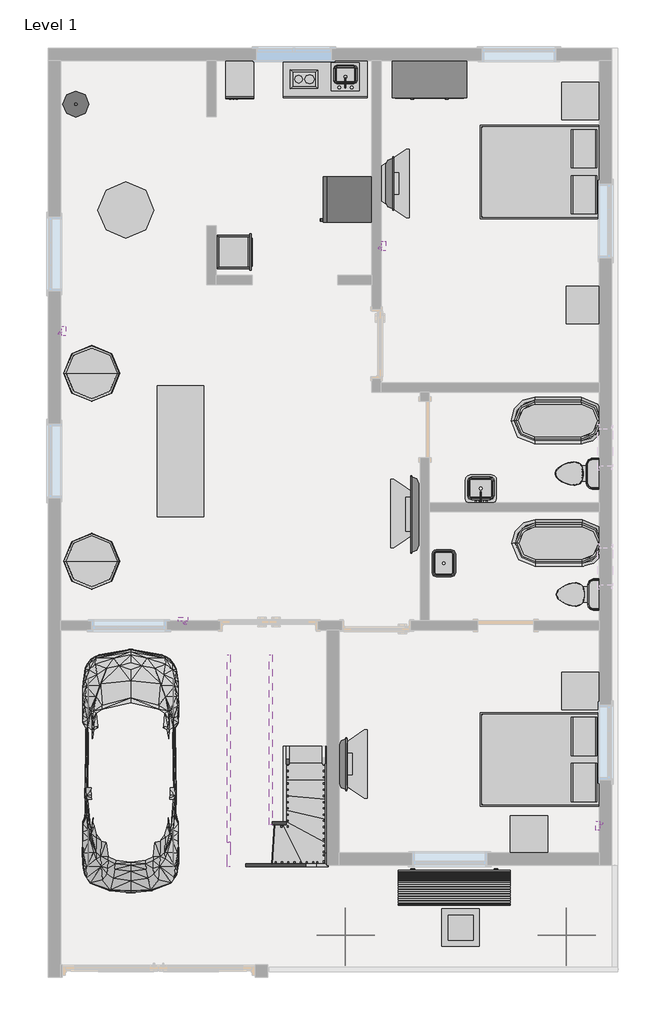
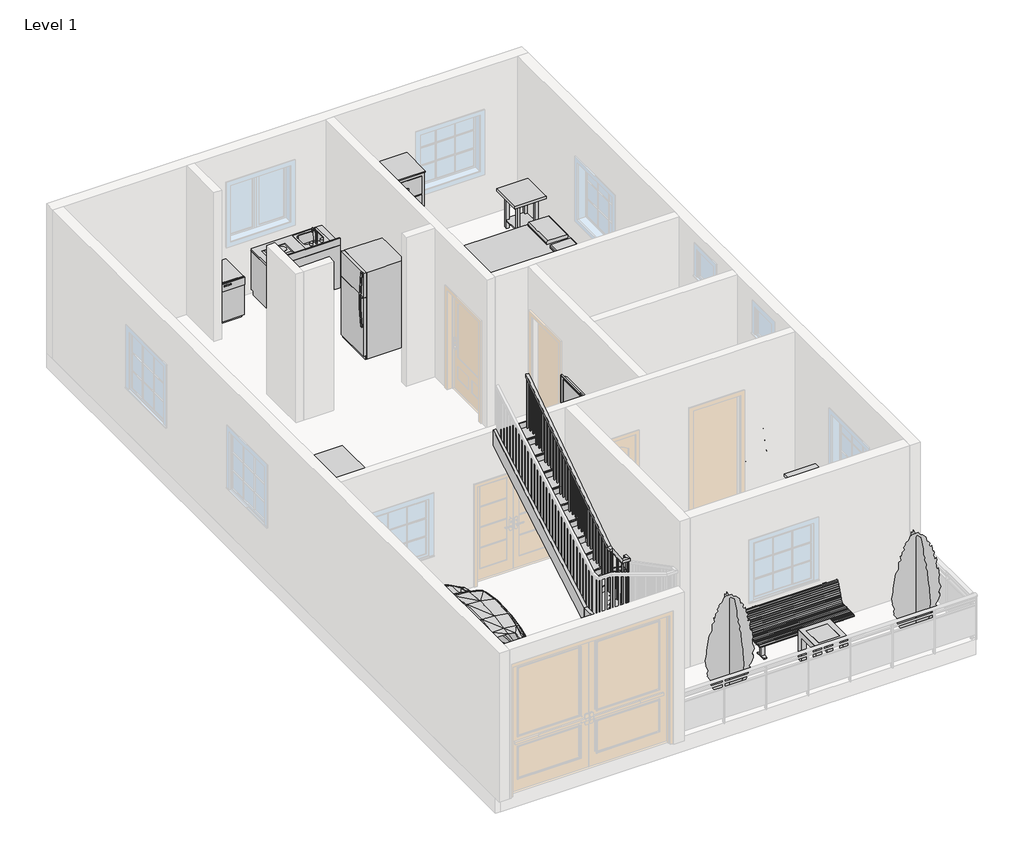
# One storey, part 3 of 3: 19 furniture elements, 10 proxies, 9 members, 8 flow terminals, 3 geographic elements, 1 railing, 1 stair flight.
"""IFC4 building model written with IfcOpenShell, lengths in millimetres."""

from ifc_helpers import new_model, si_unit, frame, origin, place, context, project, spatial, polyline, outline, extrude, faceted_brep, transform, mapped, element, save
from components import proxy_7e1014cc, proxy_fe84b772, proxy_844211aa, proxy_8b8c2dc4, rpc_beetle_rpc_beetle_3ce7ba48, rpc_picture_frame_rpc_picture_frame_c25e3fe9, proxy_a13a33b2, flow_terminal_871c2e40, flow_terminal_d49f872f, flow_terminal_62a433f7, toilet_domestic_3d_toilet_domestic_3d_f7549cf7, toilet_domestic_3d_toilet_domestic_3d_183bbd19, flow_terminal_b374fae2, furniture_1d2926bd, furniture_95afb093, furniture_9fa109b2, furniture_56245f3a, furniture_fdf74506, tv_stand_tv_stand_6ce107e5, furniture_b5c51a22, furniture_92191dda, furniture_905aceb5, furniture_5bc9ed15, furniture_c80d6d9c, geographic_element_235d1464, rpc_tree_conifer_chinese_juniper_7_1b9786cd, stair_flight_e7e63c14

model = new_model("IFC4")

# Units and contexts
model_context = context("Model", 3, world=origin())
ifc_project = project(units=[si_unit("LENGTHUNIT", "METRE", prefix="MILLI")], contexts=[model_context])

# Site, building, storey
site = spatial("IfcSite", under=ifc_project)
building = spatial("IfcBuilding", under=site)
storey = spatial("IfcBuildingStorey", under=building, Name="Level 1", Elevation=0.0)

# Proxies
placement = place(None, origin())
proxy_shape = proxy_7e1014cc(model_context)
element("IfcBuildingElementProxy", 1, Name="18\" x 24\" x 34 1/2\"", ObjectType="18\" x 24\" x 34 1/2\"", at=placement, inside=storey, context=model_context, shape_type="MappedRepresentation", body=[
    mapped(proxy_shape, transform((-12711.8273955, 12635.8692234, 0.0), x_axis=(1.0, 0.0, 0.0), y_axis=(0.0, 1.0, 0.0), z_axis=(0.0, 0.0, 1.0))),
])
proxy_2_shape = proxy_fe84b772(model_context)
element("IfcBuildingElementProxy", 2, Name="Cook Top-2 Unit : 12\" x 18\"", ObjectType="Cook Top-2 Unit : 12\" x 18\"", at=placement, inside=storey, context=model_context, shape_type="MappedRepresentation", body=[
    mapped(proxy_2_shape, transform((-11381.8347226, 12978.5187882, 0.0), x_axis=(0.0, -1.0000000000000002, 0.0), y_axis=(1.0000000000000002, 0.0, 0.0), z_axis=(0.0, 0.0, 1.0))),
])
proxy_3_shape = proxy_844211aa(model_context)
element("IfcBuildingElementProxy", 3, Name="Kitchenette - Small : 54\"", ObjectType="Kitchenette - Small : 54\"", at=placement, inside=storey, context=model_context, shape_type="MappedRepresentation", body=[
    mapped(proxy_3_shape, transform((-10989.9722221, 12597.5187882, 0.0), x_axis=(-1.0000000000000002, 0.0, 0.0), y_axis=(0.0, -1.0000000000000002, 0.0), z_axis=(0.0, 0.0, 1.0))),
])
proxy_4_shape = proxy_8b8c2dc4(model_context)
element("IfcBuildingElementProxy", 4, Name="Oven Double-Built-in : 21 1/2\" x 39 1/4\" x 21\"", ObjectType="Oven Double-Built-in : 21 1/2\" x 39 1/4\" x 21\"", at=placement, inside=storey, context=model_context, shape_type="MappedRepresentation", body=[
    mapped(proxy_4_shape, transform((-12366.2440681, 10118.0937155, 0.0), x_axis=(0.0, 1.0000000000000009, 0.0), y_axis=(-1.0000000000000009, 0.0, 0.0), z_axis=(0.0, 0.0, 1.0))),
])
rpc_beetle_rpc_beetle_shape = rpc_beetle_rpc_beetle_3ce7ba48(model_context)
element("IfcBuildingElementProxy", 5, Name="RPC Beetle : RPC Beetle", ObjectType="RPC Beetle : RPC Beetle", at=placement, inside=storey, context=model_context, shape_type="MappedRepresentation", body=[
    mapped(rpc_beetle_rpc_beetle_shape, transform((-14183.709927, 380.1187882, 0.0), x_axis=(1.0, 0.0, 0.0), y_axis=(0.0, 1.0, 0.0), z_axis=(0.0, 0.0, 1.0))),
])
rpc_picture_frame_rpc_picture_frame_shape = rpc_picture_frame_rpc_picture_frame_c25e3fe9(model_context)
element("IfcBuildingElementProxy", 6, Name="RPC Picture Frame : RPC Picture Frame", ObjectType="RPC Picture Frame : RPC Picture Frame", at=placement, inside=storey, context=model_context, shape_type="MappedRepresentation", body=[
    mapped(rpc_picture_frame_rpc_picture_frame_shape, transform((-10081.609927, 10181.9106753, 1828.8), x_axis=(0.0, 1.0000000000000002, 0.0), y_axis=(-1.0000000000000002, 0.0, 0.0), z_axis=(0.0, 0.0, 1.0))),
])
element("IfcBuildingElementProxy", 7, Name="RPC Picture Frame : RPC Picture Frame", ObjectType="RPC Picture Frame : RPC Picture Frame", at=placement, inside=storey, context=model_context, shape_type="MappedRepresentation", body=[
    mapped(rpc_picture_frame_rpc_picture_frame_shape, transform((-13328.659788, 4063.1187882, 1828.8), x_axis=(-1.0000000000000004, 0.0, 0.0), y_axis=(0.0, -1.0000000000000004, 0.0), z_axis=(0.0, 0.0, 1.0))),
])
element("IfcBuildingElementProxy", 8, Name="RPC Picture Frame : RPC Picture Frame", ObjectType="RPC Picture Frame : RPC Picture Frame", at=placement, inside=storey, context=model_context, shape_type="MappedRepresentation", body=[
    mapped(rpc_picture_frame_rpc_picture_frame_shape, transform((-6538.309927, 721.2019208, 1828.8), x_axis=(0.0, -1.0, 0.0), y_axis=(1.0, 0.0, 0.0), z_axis=(0.0, 0.0, 1.0))),
])
element("IfcBuildingElementProxy", 9, Name="RPC Picture Frame : RPC Picture Frame", ObjectType="RPC Picture Frame : RPC Picture Frame", at=placement, inside=storey, context=model_context, shape_type="MappedRepresentation", body=[
    mapped(rpc_picture_frame_rpc_picture_frame_shape, transform((-15301.309927, 8792.5721636, 1524.0), x_axis=(0.0, 1.0000000000000004, 0.0), y_axis=(-1.0000000000000004, 0.0, 0.0), z_axis=(0.0, 0.0, 1.0))),
])
proxy_5_shape = proxy_a13a33b2(model_context)
element("IfcBuildingElementProxy", 10, Name="Refrigerator : 30\" x 32\" RH", ObjectType="Refrigerator : 30\" x 32\" RH", at=placement, inside=storey, context=model_context, shape_type="MappedRepresentation", body=[
    mapped(proxy_5_shape, transform((-10619.772427, 10938.9698167, 0.0), x_axis=(0.0, -1.0000000000000007, 0.0), y_axis=(1.0000000000000007, 0.0, 0.0), z_axis=(0.0, 0.0, 1.0))),
])

# Flow terminals
flow_terminal_shape = flow_terminal_871c2e40(model_context)
element("IfcFlowTerminal", 11, ObjectType="Sink Kitchen-Island : 18\" x 18\"", at=placement, inside=storey, context=model_context, shape_type="MappedRepresentation", body=[
    mapped(flow_terminal_shape, transform((-10662.8206864, 12942.7641893, 0.0), x_axis=(-1.0000000000000002, 0.0, 0.0), y_axis=(0.0, -1.0000000000000002, 0.0), z_axis=(0.0, 0.0, 1.0))),
])
flow_terminal_2_shape = flow_terminal_d49f872f(model_context)
element("IfcFlowTerminal", 12, ObjectType="Sink Vanity-Round : 19\" x 19\"", at=placement, inside=storey, context=model_context, shape_type="MappedRepresentation", body=[
    mapped(flow_terminal_2_shape, transform((-14991.5151855, 12399.2670476, 609.6), x_axis=(0.0, 1.0000000000000002, 0.0), y_axis=(-1.0000000000000002, 0.0, 0.0), z_axis=(0.0, 0.0, 1.0))),
])
flow_terminal_3_shape = flow_terminal_62a433f7(model_context)
element("IfcFlowTerminal", 13, ObjectType="Sink Vanity-Square : 20\" x 18\"", at=placement, inside=storey, context=model_context, shape_type="MappedRepresentation", body=[
    mapped(flow_terminal_3_shape, transform((-9126.7645259, 4987.2295476, 609.6), x_axis=(0.0, 1.0000000000000002, 0.0), y_axis=(-1.0000000000000002, 0.0, 0.0), z_axis=(0.0, 0.0, 1.0))),
])
element("IfcFlowTerminal", 14, ObjectType="Sink Vanity-Square : 20\" x 18\"", at=placement, inside=storey, context=model_context, shape_type="MappedRepresentation", body=[
    mapped(flow_terminal_3_shape, transform((-8453.0206864, 6173.6641893, 0.0), x_axis=(-1.0000000000000002, 0.0, 0.0), y_axis=(0.0, -1.0000000000000002, 0.0), z_axis=(0.0, 0.0, 1.0))),
])
toilet_domestic_3d_toilet_domestic_3d_shape = toilet_domestic_3d_toilet_domestic_3d_f7549cf7(model_context)
toilet_domestic_3d_toilet_domestic_3d_2_shape = toilet_domestic_3d_toilet_domestic_3d_183bbd19(model_context)
element("IfcFlowTerminal", 15, ObjectType="Toilet-Domestic-3D : Toilet-Domestic-3D", at=placement, inside=storey, context=model_context, shape_type="MappedRepresentation", body=[
    mapped(toilet_domestic_3d_toilet_domestic_3d_shape, transform((-6931.4059544, 4494.9187882, 0.0), x_axis=(0.0, -1.0000000000000002, 0.0), y_axis=(1.0000000000000002, 0.0, 0.0), z_axis=(0.0, 0.0, 1.0))),
    mapped(toilet_domestic_3d_toilet_domestic_3d_2_shape, transform((-6931.4059544, 4494.9187882, 0.0), x_axis=(0.0, -1.0000000000000002, 0.0), y_axis=(1.0000000000000002, 0.0, 0.0), z_axis=(0.0, 0.0, 1.0))),
])
element("IfcFlowTerminal", 16, ObjectType="Toilet-Domestic-3D : Toilet-Domestic-3D", at=placement, inside=storey, context=model_context, shape_type="MappedRepresentation", body=[
    mapped(toilet_domestic_3d_toilet_domestic_3d_shape, transform((-6951.6789119, 6468.579724, 0.0), x_axis=(0.0, -1.0000000000000002, 0.0), y_axis=(1.0000000000000002, 0.0, 0.0), z_axis=(0.0, 0.0, 1.0))),
    mapped(toilet_domestic_3d_toilet_domestic_3d_2_shape, transform((-6951.6789119, 6468.579724, 0.0), x_axis=(0.0, -1.0000000000000002, 0.0), y_axis=(1.0000000000000002, 0.0, 0.0), z_axis=(0.0, 0.0, 1.0))),
])
flow_terminal_4_shape = flow_terminal_b374fae2(model_context)
element("IfcFlowTerminal", 17, ObjectType="Tub-Free Standing-3D : 30\" x 60\"", at=placement, inside=storey, context=model_context, shape_type="MappedRepresentation", body=[
    mapped(flow_terminal_4_shape, transform((-7198.709927, 5333.1187882, 0.0), x_axis=(0.0, -1.0000000000000004, 0.0), y_axis=(1.0000000000000004, 0.0, 0.0), z_axis=(0.0, 0.0, 1.0))),
])
element("IfcFlowTerminal", 18, ObjectType="Tub-Free Standing-3D : 30\" x 60\"", at=placement, inside=storey, context=model_context, shape_type="MappedRepresentation", body=[
    mapped(flow_terminal_4_shape, transform((-7212.3416169, 7332.469688, 0.0), x_axis=(0.0, -1.0000000000000004, 0.0), y_axis=(1.0000000000000004, 0.0, 0.0), z_axis=(0.0, 0.0, 1.0))),
])

# Furniture
furniture_shape = furniture_1d2926bd(model_context)
element("IfcFurniture", 19, ObjectType="Bed-Box : Queen 60\" x 79\"", at=placement, inside=storey, context=model_context, shape_type="MappedRepresentation", body=[
    mapped(furniture_shape, transform((-7243.6804188, 2141.6712472, 0.0), x_axis=(0.0, -1.0, 0.0), y_axis=(1.0, 0.0, 0.0), z_axis=(0.0, 0.0, 1.0))),
])
element("IfcFurniture", 20, ObjectType="Bed-Box : Queen 60\" x 79\"", at=placement, inside=storey, context=model_context, shape_type="MappedRepresentation", body=[
    mapped(furniture_shape, transform((-7243.6804188, 11730.1712472, 0.0), x_axis=(0.0, -1.0, 0.0), y_axis=(1.0, 0.0, 0.0), z_axis=(0.0, 0.0, 1.0))),
])
furniture_2_shape = furniture_95afb093(model_context)
element("IfcFurniture", 21, ObjectType="Counter Top w Sink Hole : 24\" Depth", at=placement, inside=storey, context=model_context, shape_type="MappedRepresentation", body=[
    mapped(furniture_2_shape, transform((-11523.3722221, 12597.5187882, 0.0), x_axis=(-1.0000000000000002, 0.0, 0.0), y_axis=(0.0, -1.0000000000000002, 0.0), z_axis=(0.0, 0.0, 1.0))),
])
furniture_3_shape = furniture_9fa109b2(model_context)
element("IfcFurniture", 22, ObjectType="Dresser : 48\" x 72\" x 24\"", at=placement, inside=storey, context=model_context, shape_type="MappedRepresentation", body=[
    mapped(furniture_3_shape, transform((-9037.7166672, 13265.4817423, 0.0), x_axis=(1.0, 0.0, 0.0), y_axis=(0.0, 1.0, 0.0), z_axis=(0.0, 0.0, 1.0))),
])
furniture_4_shape = furniture_56245f3a(model_context)
element("IfcFurniture", 23, ObjectType="TV - Flat Screen : 32\"", at=placement, inside=storey, context=model_context, shape_type="MappedRepresentation", body=[
    mapped(furniture_4_shape, transform((-9959.5713034, 11204.4633023, 914.4), x_axis=(0.0, 1.0000000000000002, 0.0), y_axis=(-1.0000000000000002, 0.0, 0.0), z_axis=(0.0, 0.0, 1.0))),
])
element("IfcFurniture", 24, ObjectType="TV - Flat Screen : 32\"", at=placement, inside=storey, context=model_context, shape_type="MappedRepresentation", body=[
    mapped(furniture_4_shape, transform((-10721.5713034, 1730.2633023, 914.4), x_axis=(0.0, 1.0000000000000002, 0.0), y_axis=(-1.0000000000000002, 0.0, 0.0), z_axis=(0.0, 0.0, 1.0))),
])
furniture_5_shape = furniture_fdf74506(model_context)
element("IfcFurniture", 25, ObjectType="TV - Flat Screen : 50\"", at=placement, inside=storey, context=model_context, shape_type="MappedRepresentation", body=[
    mapped(furniture_5_shape, transform((-9543.2485507, 5797.1321546, 914.4), x_axis=(0.0, -1.0000000000000007, 0.0), y_axis=(1.0000000000000007, 0.0, 0.0), z_axis=(0.0, 0.0, 1.0))),
])
tv_stand_tv_stand_shape = tv_stand_tv_stand_6ce107e5(model_context)
element("IfcFurniture", 26, ObjectType="TV Stand : TV Stand", at=placement, inside=storey, context=model_context, shape_type="MappedRepresentation", body=[
    mapped(tv_stand_tv_stand_shape, transform((-10094.309927, 11075.3307861, 0.0), x_axis=(0.0, 1.0000000000000002, 0.0), y_axis=(-1.0000000000000002, 0.0, 0.0), z_axis=(0.0, 0.0, 1.0))),
])
element("IfcFurniture", 27, ObjectType="TV Stand : TV Stand", at=placement, inside=storey, context=model_context, shape_type="MappedRepresentation", body=[
    mapped(tv_stand_tv_stand_shape, transform((-10780.109927, 1601.1307861, 0.0), x_axis=(0.0, 1.0000000000000002, 0.0), y_axis=(-1.0000000000000002, 0.0, 0.0), z_axis=(0.0, 0.0, 1.0))),
])
element("IfcFurniture", 28, ObjectType="TV Stand : TV Stand", at=placement, inside=storey, context=model_context, shape_type="MappedRepresentation", body=[
    mapped(tv_stand_tv_stand_shape, transform((-9484.709927, 5940.9067903, 0.0), x_axis=(0.0, -1.0000000000000007, 0.0), y_axis=(1.0000000000000007, 0.0, 0.0), z_axis=(0.0, 0.0, 1.0))),
])
furniture_6_shape = furniture_b5c51a22(model_context)
element("IfcFurniture", 29, ObjectType="Table-Coffee : 24\" x 24\" x 24\"", at=placement, inside=storey, context=model_context, shape_type="MappedRepresentation", body=[
    mapped(furniture_6_shape, transform((-8817.1756937, -1035.8922896, 0.0), x_axis=(1.0, 0.0, 0.0), y_axis=(0.0, 1.0, 0.0), z_axis=(0.0, 0.0, 1.0))),
])
furniture_7_shape = furniture_92191dda(model_context)
element("IfcFurniture", 30, ObjectType="Table-Dining : 30\" x 84\" x 22\"", at=placement, inside=storey, context=model_context, shape_type="MappedRepresentation", body=[
    mapped(furniture_7_shape, transform((-13275.6988492, 6813.4530215, 0.0), x_axis=(0.0, 1.0, 0.0), y_axis=(-1.0, 0.0, 0.0), z_axis=(0.0, 0.0, 1.0))),
])
furniture_8_shape = furniture_905aceb5(model_context)
element("IfcFurniture", 31, ObjectType="Table-Dining Round w Chairs : 36\" Diameter", at=placement, inside=storey, context=model_context, shape_type="MappedRepresentation", body=[
    mapped(furniture_8_shape, transform((-14363.5918942, 10953.5974767, 0.0), x_axis=(1.0, 0.0, 0.0), y_axis=(0.0, 1.0, 0.0), z_axis=(0.0, 0.0, 1.0))),
])
furniture_9_shape = furniture_5bc9ed15(model_context)
element("IfcFurniture", 32, ObjectType="Table-Night Stand : 24\" x 24\" x 30\"", at=placement, inside=storey, context=model_context, shape_type="MappedRepresentation", body=[
    mapped(furniture_9_shape, transform((-7989.8435573, 278.5187882, 0.0), x_axis=(1.0, 0.0, 0.0), y_axis=(0.0, 1.0, 0.0), z_axis=(0.0, 0.0, 1.0))),
])
element("IfcFurniture", 33, ObjectType="Table-Night Stand : 24\" x 24\" x 30\"", at=placement, inside=storey, context=model_context, shape_type="MappedRepresentation", body=[
    mapped(furniture_9_shape, transform((-7151.6435573, 2615.3187882, 0.0), x_axis=(1.0, 0.0, 0.0), y_axis=(0.0, 1.0, 0.0), z_axis=(0.0, 0.0, 1.0))),
])
element("IfcFurniture", 34, ObjectType="Table-Night Stand : 24\" x 24\" x 30\"", at=placement, inside=storey, context=model_context, shape_type="MappedRepresentation", body=[
    mapped(furniture_9_shape, transform((-7075.4435573, 8914.5187882, 0.0), x_axis=(1.0, 0.0, 0.0), y_axis=(0.0, 1.0, 0.0), z_axis=(0.0, 0.0, 1.0))),
])
element("IfcFurniture", 35, ObjectType="Table-Night Stand : 24\" x 24\" x 30\"", at=placement, inside=storey, context=model_context, shape_type="MappedRepresentation", body=[
    mapped(furniture_9_shape, transform((-7151.6435573, 12241.9187882, 0.0), x_axis=(1.0, 0.0, 0.0), y_axis=(0.0, 1.0, 0.0), z_axis=(0.0, 0.0, 1.0))),
])
furniture_10_shape = furniture_c80d6d9c(model_context)
element("IfcFurniture", 36, ObjectType="Table-Round : 36\" Diameter", at=placement, inside=storey, context=model_context, shape_type="MappedRepresentation", body=[
    mapped(furniture_10_shape, transform((-14818.709927, 5034.6687882, 0.0), x_axis=(1.0, 0.0, 0.0), y_axis=(0.0, 1.0, 0.0), z_axis=(0.0, 0.0, 1.0))),
])
element("IfcFurniture", 37, ObjectType="Table-Round : 36\" Diameter", at=placement, inside=storey, context=model_context, shape_type="MappedRepresentation", body=[
    mapped(furniture_10_shape, transform((-14818.709927, 8101.7187882, 0.0), x_axis=(1.0, 0.0, 0.0), y_axis=(0.0, 1.0, 0.0), z_axis=(0.0, 0.0, 1.0))),
])

# Geographic elements
geographic_element_shape = geographic_element_235d1464(model_context)
element("IfcGeographicElement", 38, ObjectType="Park Bench : 72\"", at=placement, inside=storey, context=model_context, shape_type="MappedRepresentation", body=[
    mapped(geographic_element_shape, transform((-8900.509927, -254.8812118, 0.0), x_axis=(1.0, 0.0, 0.0), y_axis=(0.0, 1.0, 0.0), z_axis=(0.0, 0.0, 1.0))),
])
rpc_tree_conifer_chinese_juniper_7_shape = rpc_tree_conifer_chinese_juniper_7_1b9786cd(model_context)
element("IfcGeographicElement", 39, ObjectType="RPC Tree - Conifer : Chinese Juniper - 7'", at=placement, inside=storey, context=model_context, shape_type="MappedRepresentation", body=[
    mapped(rpc_tree_conifer_chinese_juniper_7_shape, transform((-7071.9065981, -1067.6812118, 0.0), x_axis=(1.0, 0.0, 0.0), y_axis=(0.0, 1.0, 0.0), z_axis=(0.0, 0.0, 1.0))),
])
element("IfcGeographicElement", 40, ObjectType="RPC Tree - Conifer : Chinese Juniper - 7'", at=placement, inside=storey, context=model_context, shape_type="MappedRepresentation", body=[
    mapped(rpc_tree_conifer_chinese_juniper_7_shape, transform((-10678.7065981, -1067.6812118, 0.0), x_axis=(1.0, 0.0, 0.0), y_axis=(0.0, 1.0, 0.0), z_axis=(0.0, 0.0, 1.0))),
])

# Members
element("IfcMember", 41, ObjectType="Stringer - 2\" Width", at=placement, inside=storey, context=model_context, shape_type="SweptSolid", body=[
    extrude(outline(polyline([(2021.0747681, 228.2877104), (2021.0747681, 0.0), (1799.7506701, 0.0), (282.218871, 792.3221478), (282.218871, 1136.165911), (2021.0747681, 228.2877104)])), frame((-11008.709927, 0.0, 0.0), z_axis=(1.0, 0.0, 0.0), x_axis=(0.0, 1.0, 0.0)), (0.0, 0.0, 1.0), 50.8),
])
element("IfcMember", 42, ObjectType="Stringer - 2\" Width", at=placement, inside=storey, context=model_context, shape_type="SweptSolid", body=[
    extrude(outline(polyline([(-11008.709927, 282.218871), (-10957.909927, 282.218871), (-10957.909927, 49.9187882), (-11008.709927, 100.7187882), (-11008.709927, 282.218871)])), frame((0.0, 0.0, 792.3221478), z_axis=(0.0, 0.0, 1.0), x_axis=(1.0, 0.0, 0.0)), (0.0, 0.0, 1.0), 343.8437632),
])
element("IfcMember", 43, ObjectType="Stringer - 2\" Width", at=placement, inside=storey, context=model_context, shape_type="SweptSolid", body=[
    extrude(outline(polyline([(-11008.709927, 100.7187882), (-10957.909927, 49.9187882), (-11146.1388782, 49.9187882), (-11146.1388782, 100.7187882), (-11008.709927, 100.7187882)])), frame((0.0, 0.0, 792.3221478), z_axis=(0.0, 0.0, 1.0), x_axis=(1.0, 0.0, 0.0)), (0.0, 0.0, 1.0), 343.8437632),
])
element("IfcMember", 44, ObjectType="Stringer - 2\" Width", at=placement, inside=storey, context=model_context, shape_type="SweptSolid", body=[
    extrude(outline(polyline([(792.3221478, -11146.1388782), (1136.165911, -11146.1388782), (1622.0745047, -12526.8544326), (1622.0745047, -12558.109927), (1289.2303375, -12558.109927), (792.3221478, -11146.1388782)])), frame((0.0, 49.9187882, 0.0), z_axis=(0.0, 1.0, 0.0), x_axis=(0.0, 0.0, 1.0)), (0.0, 0.0, 1.0), 50.8),
])
element("IfcMember", 45, ObjectType="Stringer - 2\" Width", at=placement, inside=storey, context=model_context, shape_type="SweptSolid", body=[
    extrude(outline(polyline([(-12558.109927, 49.9187882), (-12608.909927, 49.9187882), (-12608.909927, 452.8070148), (-12558.109927, 452.8070148), (-12558.109927, 49.9187882)])), frame((0.0, 0.0, 1298.95037), z_axis=(0.0, 0.0, 1.0), x_axis=(1.0, 0.0, 0.0)), (0.0, 0.0, 1.0), 323.1241347),
])
element("IfcMember", 46, ObjectType="Stringer - 2\" Width", at=placement, inside=storey, context=model_context, shape_type="SweptSolid", body=[
    extrude(outline(polyline([(2021.0747681, 194.0438558), (2021.0747681, 0.0), (1767.5677761, 0.0), (786.5187882, 693.7300285), (786.5187882, 1067.0365052), (2021.0747681, 194.0438558)])), frame((-11694.509927, 0.0, 0.0), z_axis=(1.0, 0.0, 0.0), x_axis=(0.0, 1.0, 0.0)), (0.0, 0.0, 1.0), 50.8),
])
element("IfcMember", 47, ObjectType="Stringer - 2\" Width", at=placement, inside=storey, context=model_context, shape_type="SweptSolid", body=[
    extrude(outline(polyline([(729.6522769, -11643.709927), (1279.6063607, -11643.709927), (1569.0312677, -11828.841892), (1569.0312677, -11872.309927), (1071.3347916, -11872.309927), (729.6522769, -11653.7511444), (729.6522769, -11643.709927)])), frame((0.0, 735.7187882, 0.0), z_axis=(0.0, 1.0, 0.0), x_axis=(0.0, 0.0, 1.0)), (0.0, 0.0, 1.0), 50.8),
])
element("IfcMember", 48, ObjectType="Stringer - 2\" Width", at=placement, inside=storey, context=model_context, shape_type="SweptSolid", body=[
    extrude(outline(polyline([(735.7187882, 1200.3198695), (735.7187882, 1569.0312677), (3510.3281176, 3457.6683543), (3510.3281176, 3088.9569562), (735.7187882, 1200.3198695)])), frame((-11923.109927, 0.0, 0.0), z_axis=(1.0, 0.0, 0.0), x_axis=(0.0, 1.0, 0.0)), (0.0, 0.0, 1.0), 50.8),
])
element("IfcMember", 49, ObjectType="Stringer - 2\" Width", at=placement, inside=storey, context=model_context, shape_type="SweptSolid", body=[
    extrude(outline(polyline([(452.8070148, 1298.95037), (452.8070148, 1622.0745047), (3510.3281176, 3404.7346341), (3510.3281176, 3081.6104994), (452.8070148, 1298.95037)])), frame((-12608.909927, 0.0, 0.0), z_axis=(1.0, 0.0, 0.0), x_axis=(0.0, 1.0, 0.0)), (0.0, 0.0, 1.0), 50.8),
])

# Railing
element("IfcRailing", 50, ObjectType="Handrail - Rectangular", at=placement, inside=storey, context=model_context, shape_type="SolidModel", body=[
    faceted_brep([(-11592.909927, 2021.0747681, 1055.4943004), (-11592.909927, 2021.0747681, 993.2765543), (-11643.709927, 2021.0747681, 993.2765543), (-11643.709927, 2021.0747681, 1055.4943004), (-11592.909927, 811.9187882, 1910.5258256), (-11592.909927, 761.1187882, 1884.2303279), (-11643.709927, 761.1187882, 1884.2303279), (-11643.709927, 811.9187882, 1910.5258256), (-11592.909927, 811.9187882, 2135.0948552), (-11592.909927, 761.1187882, 2084.2948552), (-11643.709927, 761.1187882, 2084.2948552), (-11643.709927, 811.9187882, 2135.0948552), (-11592.909927, 684.9187882, 2135.0948552), (-11592.909927, 684.9187882, 2084.2948552), (-11643.709927, 735.7187882, 2084.2948552), (-11643.709927, 735.7187882, 2135.0948552), (-11719.909927, 684.9187882, 2135.0948552), (-11747.7191183, 684.9187882, 2084.2948552), (-11747.7191183, 735.7187882, 2084.2948552), (-11719.909927, 735.7187882, 2135.0948552), (-11923.109927, 684.9187882, 2452.7663124), (-11923.109927, 735.7187882, 2452.7663124), (-11923.109927, 735.7187882, 2358.490986), (-11923.109927, 684.9187882, 2358.490986)], [[[0, 1, 2, 3]], [[1, 0, 4, 5]], [[2, 1, 5, 6]], [[3, 2, 6, 7]], [[0, 3, 7, 4]], [[5, 4, 8, 9]], [[6, 5, 9, 10]], [[7, 6, 10, 11]], [[4, 7, 11, 8]], [[9, 8, 12, 13]], [[10, 9, 13, 14]], [[11, 10, 14, 15]], [[8, 11, 15, 12]], [[13, 12, 16, 17]], [[14, 13, 17, 18]], [[15, 14, 18, 19]], [[12, 15, 19, 16]], [[20, 21, 22, 23]], [[17, 16, 20, 23]], [[18, 17, 23, 22]], [[19, 18, 22, 21]], [[16, 19, 21, 20]]]),
    faceted_brep([(-11973.909927, 684.9187882, 2454.2328383), (-11973.909927, 684.9187882, 2403.4328383), (-11923.109927, 684.9187882, 2403.4328383), (-11923.109927, 684.9187882, 2454.2328383), (-11973.909927, 766.500962, 2454.2328383), (-11973.909927, 782.1497388, 2403.4328383), (-11923.109927, 782.1497388, 2403.4328383), (-11923.109927, 766.500962, 2454.2328383), (-11973.909927, 3510.3281176, 4321.9169374), (-11923.109927, 3510.3281176, 4321.9169374), (-11923.109927, 3510.3281176, 4260.4650377), (-11973.909927, 3510.3281176, 4260.4650377)], [[[0, 1, 2, 3]], [[1, 0, 4, 5]], [[2, 1, 5, 6]], [[3, 2, 6, 7]], [[0, 3, 7, 4]], [[8, 9, 10, 11]], [[5, 4, 8, 11]], [[6, 5, 11, 10]], [[7, 6, 10, 9]], [[4, 7, 9, 8]]]),
    extrude(outline(polyline([(3500.175962, 4253.5546098), (3519.225962, 4266.5216737), (3519.225962, 3217.3333333), (3500.175962, 3217.3333333), (3500.175962, 4253.5546098)])), frame((-11958.034927, 0.0, 0.0), z_axis=(1.0, 0.0, 0.0), x_axis=(0.0, 1.0, 0.0)), (0.0, 0.0, 1.0), 19.05),
    extrude(outline(polyline([(3398.575962, 4184.3969356), (3417.625962, 4197.3639995), (3417.625962, 3217.3333333), (3398.575962, 3217.3333333), (3398.575962, 4184.3969356)])), frame((-11958.034927, 0.0, 0.0), z_axis=(1.0, 0.0, 0.0), x_axis=(0.0, 1.0, 0.0)), (0.0, 0.0, 1.0), 19.05),
    extrude(outline(polyline([(3296.975962, 4115.2392614), (3316.025962, 4128.2063254), (3316.025962, 3217.3333333), (3296.975962, 3217.3333333), (3296.975962, 4115.2392614)])), frame((-11958.034927, 0.0, 0.0), z_axis=(1.0, 0.0, 0.0), x_axis=(0.0, 1.0, 0.0)), (0.0, 0.0, 1.0), 19.05),
    extrude(outline(polyline([(3195.375962, 4046.0815873), (3214.425962, 4059.0486512), (3214.425962, 3048.0), (3195.375962, 3048.0), (3195.375962, 4046.0815873)])), frame((-11958.034927, 0.0, 0.0), z_axis=(1.0, 0.0, 0.0), x_axis=(0.0, 1.0, 0.0)), (0.0, 0.0, 1.0), 19.05),
    extrude(outline(polyline([(3093.775962, 3976.9239131), (3112.825962, 3989.890977), (3112.825962, 3048.0), (3093.775962, 3048.0), (3093.775962, 3976.9239131)])), frame((-11958.034927, 0.0, 0.0), z_axis=(1.0, 0.0, 0.0), x_axis=(0.0, 1.0, 0.0)), (0.0, 0.0, 1.0), 19.05),
    extrude(outline(polyline([(2992.175962, 3907.7662389), (3011.225962, 3920.7333028), (3011.225962, 3048.0), (2992.175962, 3048.0), (2992.175962, 3907.7662389)])), frame((-11958.034927, 0.0, 0.0), z_axis=(1.0, 0.0, 0.0), x_axis=(0.0, 1.0, 0.0)), (0.0, 0.0, 1.0), 19.05),
    extrude(outline(polyline([(2890.575962, 3838.6085647), (2909.625962, 3851.5756286), (2909.625962, 2878.6666667), (2890.575962, 2878.6666667), (2890.575962, 3838.6085647)])), frame((-11958.034927, 0.0, 0.0), z_axis=(1.0, 0.0, 0.0), x_axis=(0.0, 1.0, 0.0)), (0.0, 0.0, 1.0), 19.05),
    extrude(outline(polyline([(2788.975962, 3769.4508905), (2808.025962, 3782.4179544), (2808.025962, 2878.6666667), (2788.975962, 2878.6666667), (2788.975962, 3769.4508905)])), frame((-11958.034927, 0.0, 0.0), z_axis=(1.0, 0.0, 0.0), x_axis=(0.0, 1.0, 0.0)), (0.0, 0.0, 1.0), 19.05),
    extrude(outline(polyline([(2687.375962, 3700.2932163), (2706.425962, 3713.2602802), (2706.425962, 2878.6666667), (2687.375962, 2878.6666667), (2687.375962, 3700.2932163)])), frame((-11958.034927, 0.0, 0.0), z_axis=(1.0, 0.0, 0.0), x_axis=(0.0, 1.0, 0.0)), (0.0, 0.0, 1.0), 19.05),
    extrude(outline(polyline([(2585.775962, 3631.1355421), (2604.825962, 3644.102606), (2604.825962, 2709.3333333), (2585.775962, 2709.3333333), (2585.775962, 3631.1355421)])), frame((-11958.034927, 0.0, 0.0), z_axis=(1.0, 0.0, 0.0), x_axis=(0.0, 1.0, 0.0)), (0.0, 0.0, 1.0), 19.05),
    extrude(outline(polyline([(2484.175962, 3561.9778679), (2503.225962, 3574.9449318), (2503.225962, 2709.3333333), (2484.175962, 2709.3333333), (2484.175962, 3561.9778679)])), frame((-11958.034927, 0.0, 0.0), z_axis=(1.0, 0.0, 0.0), x_axis=(0.0, 1.0, 0.0)), (0.0, 0.0, 1.0), 19.05),
    extrude(outline(polyline([(2382.575962, 3492.8201937), (2401.625962, 3505.7872576), (2401.625962, 2540.0), (2382.575962, 2540.0), (2382.575962, 3492.8201937)])), frame((-11958.034927, 0.0, 0.0), z_axis=(1.0, 0.0, 0.0), x_axis=(0.0, 1.0, 0.0)), (0.0, 0.0, 1.0), 19.05),
    extrude(outline(polyline([(2280.975962, 3423.6625195), (2300.025962, 3436.6295835), (2300.025962, 2540.0), (2280.975962, 2540.0), (2280.975962, 3423.6625195)])), frame((-11958.034927, 0.0, 0.0), z_axis=(1.0, 0.0, 0.0), x_axis=(0.0, 1.0, 0.0)), (0.0, 0.0, 1.0), 19.05),
    extrude(outline(polyline([(2179.375962, 3354.5048454), (2198.425962, 3367.4719093), (2198.425962, 2540.0), (2179.375962, 2540.0), (2179.375962, 3354.5048454)])), frame((-11958.034927, 0.0, 0.0), z_axis=(1.0, 0.0, 0.0), x_axis=(0.0, 1.0, 0.0)), (0.0, 0.0, 1.0), 19.05),
    extrude(outline(polyline([(2077.775962, 3285.3471712), (2096.825962, 3298.3142351), (2096.825962, 2370.6666667), (2077.775962, 2370.6666667), (2077.775962, 3285.3471712)])), frame((-11958.034927, 0.0, 0.0), z_axis=(1.0, 0.0, 0.0), x_axis=(0.0, 1.0, 0.0)), (0.0, 0.0, 1.0), 19.05),
    extrude(outline(polyline([(1976.175962, 3216.189497), (1995.225962, 3229.1565609), (1995.225962, 2370.6666667), (1976.175962, 2370.6666667), (1976.175962, 3216.189497)])), frame((-11958.034927, 0.0, 0.0), z_axis=(1.0, 0.0, 0.0), x_axis=(0.0, 1.0, 0.0)), (0.0, 0.0, 1.0), 19.05),
    extrude(outline(polyline([(1874.575962, 3147.0318228), (1893.625962, 3159.9988867), (1893.625962, 2370.6666667), (1874.575962, 2370.6666667), (1874.575962, 3147.0318228)])), frame((-11958.034927, 0.0, 0.0), z_axis=(1.0, 0.0, 0.0), x_axis=(0.0, 1.0, 0.0)), (0.0, 0.0, 1.0), 19.05),
    extrude(outline(polyline([(1772.975962, 3077.8741486), (1792.025962, 3090.8412125), (1792.025962, 2201.3333333), (1772.975962, 2201.3333333), (1772.975962, 3077.8741486)])), frame((-11958.034927, 0.0, 0.0), z_axis=(1.0, 0.0, 0.0), x_axis=(0.0, 1.0, 0.0)), (0.0, 0.0, 1.0), 19.05),
    extrude(outline(polyline([(1671.375962, 3008.7164744), (1690.425962, 3021.6835383), (1690.425962, 2201.3333333), (1671.375962, 2201.3333333), (1671.375962, 3008.7164744)])), frame((-11958.034927, 0.0, 0.0), z_axis=(1.0, 0.0, 0.0), x_axis=(0.0, 1.0, 0.0)), (0.0, 0.0, 1.0), 19.05),
    extrude(outline(polyline([(1569.775962, 2939.5588002), (1588.825962, 2952.5258641), (1588.825962, 2201.3333333), (1569.775962, 2201.3333333), (1569.775962, 2939.5588002)])), frame((-11958.034927, 0.0, 0.0), z_axis=(1.0, 0.0, 0.0), x_axis=(0.0, 1.0, 0.0)), (0.0, 0.0, 1.0), 19.05),
    extrude(outline(polyline([(1468.175962, 2870.401126), (1487.225962, 2883.3681899), (1487.225962, 2032.0), (1468.175962, 2032.0), (1468.175962, 2870.401126)])), frame((-11958.034927, 0.0, 0.0), z_axis=(1.0, 0.0, 0.0), x_axis=(0.0, 1.0, 0.0)), (0.0, 0.0, 1.0), 19.05),
    extrude(outline(polyline([(1366.575962, 2801.2434518), (1385.625962, 2814.2105157), (1385.625962, 2032.0), (1366.575962, 2032.0), (1366.575962, 2801.2434518)])), frame((-11958.034927, 0.0, 0.0), z_axis=(1.0, 0.0, 0.0), x_axis=(0.0, 1.0, 0.0)), (0.0, 0.0, 1.0), 19.05),
    extrude(outline(polyline([(1264.975962, 2732.0857776), (1284.025962, 2745.0528416), (1284.025962, 1862.6666667), (1264.975962, 1862.6666667), (1264.975962, 2732.0857776)])), frame((-11958.034927, 0.0, 0.0), z_axis=(1.0, 0.0, 0.0), x_axis=(0.0, 1.0, 0.0)), (0.0, 0.0, 1.0), 19.05),
    extrude(outline(polyline([(1163.375962, 2662.9281035), (1182.425962, 2675.8951674), (1182.425962, 1862.6666667), (1163.375962, 1862.6666667), (1163.375962, 2662.9281035)])), frame((-11958.034927, 0.0, 0.0), z_axis=(1.0, 0.0, 0.0), x_axis=(0.0, 1.0, 0.0)), (0.0, 0.0, 1.0), 19.05),
    extrude(outline(polyline([(1061.775962, 2593.7704293), (1080.825962, 2606.7374932), (1080.825962, 1862.6666667), (1061.775962, 1862.6666667), (1061.775962, 2593.7704293)])), frame((-11958.034927, 0.0, 0.0), z_axis=(1.0, 0.0, 0.0), x_axis=(0.0, 1.0, 0.0)), (0.0, 0.0, 1.0), 19.05),
    extrude(outline(polyline([(960.175962, 2524.6127551), (979.225962, 2537.579819), (979.225962, 1693.3333333), (960.175962, 1693.3333333), (960.175962, 2524.6127551)])), frame((-11958.034927, 0.0, 0.0), z_axis=(1.0, 0.0, 0.0), x_axis=(0.0, 1.0, 0.0)), (0.0, 0.0, 1.0), 19.05),
    extrude(outline(polyline([(858.575962, 2455.4550809), (877.625962, 2468.4221448), (877.625962, 1693.3333333), (858.575962, 1693.3333333), (858.575962, 2455.4550809)])), frame((-11958.034927, 0.0, 0.0), z_axis=(1.0, 0.0, 0.0), x_axis=(0.0, 1.0, 0.0)), (0.0, 0.0, 1.0), 19.05),
    extrude(outline(polyline([(2187.8200057, -11813.9394542), (2217.6017048, -11832.9894542), (1354.6666667, -11832.9894542), (1354.6666667, -11813.9394542), (2187.8200057, -11813.9394542)])), frame((0.0, 700.7937882, 0.0), z_axis=(0.0, 1.0, 0.0), x_axis=(0.0, 0.0, 1.0)), (0.0, 0.0, 1.0), 19.05),
    extrude(outline(polyline([(2028.9842771, -11712.3394542), (2058.7659762, -11731.3894542), (1185.3333333, -11731.3894542), (1185.3333333, -11712.3394542), (2028.9842771, -11712.3394542)])), frame((0.0, 700.7937882, 0.0), z_axis=(0.0, 1.0, 0.0), x_axis=(0.0, 0.0, 1.0)), (0.0, 0.0, 1.0), 19.05),
    extrude(outline(polyline([(792.3497681, 1862.1459378), (811.3997681, 1848.6750946), (811.3997681, 846.6666667), (792.3497681, 846.6666667), (792.3497681, 1862.1459378)])), frame((-11627.834927, 0.0, 0.0), z_axis=(1.0, 0.0, 0.0), x_axis=(0.0, 1.0, 0.0)), (0.0, 0.0, 1.0), 19.05),
    extrude(outline(polyline([(893.9497681, 1790.3014409), (912.9997681, 1776.8305978), (912.9997681, 846.6666667), (893.9497681, 846.6666667), (893.9497681, 1790.3014409)])), frame((-11627.834927, 0.0, 0.0), z_axis=(1.0, 0.0, 0.0), x_axis=(0.0, 1.0, 0.0)), (0.0, 0.0, 1.0), 19.05),
    extrude(outline(polyline([(995.5497681, 1718.4569441), (1014.5997681, 1704.986101), (1014.5997681, 677.3333333), (995.5497681, 677.3333333), (995.5497681, 1718.4569441)])), frame((-11627.834927, 0.0, 0.0), z_axis=(1.0, 0.0, 0.0), x_axis=(0.0, 1.0, 0.0)), (0.0, 0.0, 1.0), 19.05),
    extrude(outline(polyline([(1097.1497681, 1646.6124473), (1116.1997681, 1633.1416041), (1116.1997681, 677.3333333), (1097.1497681, 677.3333333), (1097.1497681, 1646.6124473)])), frame((-11627.834927, 0.0, 0.0), z_axis=(1.0, 0.0, 0.0), x_axis=(0.0, 1.0, 0.0)), (0.0, 0.0, 1.0), 19.05),
    extrude(outline(polyline([(1198.7497681, 1574.7679505), (1217.7997681, 1561.2971073), (1217.7997681, 508.0), (1198.7497681, 508.0), (1198.7497681, 1574.7679505)])), frame((-11627.834927, 0.0, 0.0), z_axis=(1.0, 0.0, 0.0), x_axis=(0.0, 1.0, 0.0)), (0.0, 0.0, 1.0), 19.05),
    extrude(outline(polyline([(1300.3497681, 1502.9234536), (1319.3997681, 1489.4526105), (1319.3997681, 508.0), (1300.3497681, 508.0), (1300.3497681, 1502.9234536)])), frame((-11627.834927, 0.0, 0.0), z_axis=(1.0, 0.0, 0.0), x_axis=(0.0, 1.0, 0.0)), (0.0, 0.0, 1.0), 19.05),
    extrude(outline(polyline([(1401.9497681, 1431.0789568), (1420.9997681, 1417.6081137), (1420.9997681, 508.0), (1401.9497681, 508.0), (1401.9497681, 1431.0789568)])), frame((-11627.834927, 0.0, 0.0), z_axis=(1.0, 0.0, 0.0), x_axis=(0.0, 1.0, 0.0)), (0.0, 0.0, 1.0), 19.05),
    extrude(outline(polyline([(1503.5497681, 1359.23446), (1522.5997681, 1345.7636168), (1522.5997681, 338.6666667), (1503.5497681, 338.6666667), (1503.5497681, 1359.23446)])), frame((-11627.834927, 0.0, 0.0), z_axis=(1.0, 0.0, 0.0), x_axis=(0.0, 1.0, 0.0)), (0.0, 0.0, 1.0), 19.05),
    extrude(outline(polyline([(1605.1497681, 1287.3899632), (1624.1997681, 1273.91912), (1624.1997681, 338.6666667), (1605.1497681, 338.6666667), (1605.1497681, 1287.3899632)])), frame((-11627.834927, 0.0, 0.0), z_axis=(1.0, 0.0, 0.0), x_axis=(0.0, 1.0, 0.0)), (0.0, 0.0, 1.0), 19.05),
    extrude(outline(polyline([(1706.7497681, 1215.5454663), (1725.7997681, 1202.0746232), (1725.7997681, 338.6666667), (1706.7497681, 338.6666667), (1706.7497681, 1215.5454663)])), frame((-11627.834927, 0.0, 0.0), z_axis=(1.0, 0.0, 0.0), x_axis=(0.0, 1.0, 0.0)), (0.0, 0.0, 1.0), 19.05),
    extrude(outline(polyline([(1808.3497681, 1143.7009695), (1827.3997681, 1130.2301264), (1827.3997681, 169.3333333), (1808.3497681, 169.3333333), (1808.3497681, 1143.7009695)])), frame((-11627.834927, 0.0, 0.0), z_axis=(1.0, 0.0, 0.0), x_axis=(0.0, 1.0, 0.0)), (0.0, 0.0, 1.0), 19.05),
    extrude(outline(polyline([(1909.9497681, 1071.8564727), (1928.9997681, 1058.3856295), (1928.9997681, 169.3333333), (1909.9497681, 169.3333333), (1909.9497681, 1071.8564727)])), frame((-11627.834927, 0.0, 0.0), z_axis=(1.0, 0.0, 0.0), x_axis=(0.0, 1.0, 0.0)), (0.0, 0.0, 1.0), 19.05),
    extrude(outline(polyline([(-11938.984927, 756.975962), (-11958.034927, 756.975962), (-11958.034927, 776.025962), (-11938.984927, 776.025962), (-11938.984927, 756.975962)])), frame((0.0, 0.0, 1524.0), z_axis=(0.0, 0.0, 1.0), x_axis=(1.0, 0.0, 0.0)), (0.0, 0.0, 1.0), 879.4328383),
    extrude(outline(polyline([(2383.3090686, -11938.984927), (2413.0907677, -11958.034927), (1524.0, -11958.034927), (1524.0, -11938.984927), (2383.3090686, -11938.984927)])), frame((0.0, 700.7937882, 0.0), z_axis=(0.0, 1.0, 0.0), x_axis=(0.0, 0.0, 1.0)), (0.0, 0.0, 1.0), 19.05),
    extrude(outline(polyline([(2345.0666624, -11914.522997), (2374.8483615, -11933.572997), (1354.6666667, -11933.572997), (1354.6666667, -11914.522997), (2345.0666624, -11914.522997)])), frame((0.0, 700.7937882, 0.0), z_axis=(0.0, 1.0, 0.0), x_axis=(0.0, 0.0, 1.0)), (0.0, 0.0, 1.0), 19.05),
    extrude(outline(polyline([(-11610.7394542, 719.8437882), (-11610.7394542, 700.7937882), (-11629.7894542, 700.7937882), (-11629.7894542, 719.8437882), (-11610.7394542, 719.8437882)])), frame((0.0, 0.0, 1016.0), z_axis=(0.0, 0.0, 1.0), x_axis=(1.0, 0.0, 0.0)), (0.0, 0.0, 1.0), 1068.2948552),
    extrude(outline(polyline([(-11627.834927, 719.8437882), (-11608.784927, 719.8437882), (-11608.784927, 700.7937882), (-11627.834927, 700.7937882), (-11627.834927, 719.8437882)])), frame((0.0, 0.0, 1016.0), z_axis=(0.0, 0.0, 1.0), x_axis=(1.0, 0.0, 0.0)), (0.0, 0.0, 1.0), 1068.2948552),
    extrude(outline(polyline([(-11627.834927, 724.1649089), (-11608.784927, 724.1649089), (-11608.784927, 705.1149089), (-11627.834927, 705.1149089), (-11627.834927, 724.1649089)])), frame((0.0, 0.0, 1016.0), z_axis=(0.0, 0.0, 1.0), x_axis=(1.0, 0.0, 0.0)), (0.0, 0.0, 1.0), 1068.2948552),
    extrude(outline(polyline([(3491.2781176, 4247.4979738), (3510.3281176, 4260.4650377), (3510.3281176, 3217.3333333), (3491.2781176, 3217.3333333), (3491.2781176, 4247.4979738)])), frame((-11958.034927, 0.0, 0.0), z_axis=(1.0, 0.0, 0.0), x_axis=(0.0, 1.0, 0.0)), (0.0, 0.0, 1.0), 19.05),
    extrude(outline(polyline([(2002.0247681, 1006.7473974), (2021.0747681, 993.2765543), (2021.0747681, 169.3333333), (2002.0247681, 169.3333333), (2002.0247681, 1006.7473974)])), frame((-11627.834927, 0.0, 0.0), z_axis=(1.0, 0.0, 0.0), x_axis=(0.0, 1.0, 0.0)), (0.0, 0.0, 1.0), 19.05),
])

# Stair flight
stair_flight_shape = stair_flight_e7e63c14(model_context)
element("IfcStairFlight", 51, ObjectType="2\" Tread 1\" Nosing 1/4\" Riser", at=placement, inside=storey, context=model_context, shape_type="MappedRepresentation", body=[
    mapped(stair_flight_shape, transform((0.0, 0.0, 0.0), x_axis=(1.0, 0.0, 0.0), y_axis=(0.0, 1.0, 0.0), z_axis=(0.0, 0.0, 1.0))),
])

save(model, "model.ifc")

# Revit data of these elements
# Type "18\" x 24\" x 34 1/2\""
#   Label = "T"
#   Assembly Code = "E1090400"
#   Depth = 2' - 0"
#   Height = 2' - 10 1/2"
#   Width = 1' - 6"
#   Panel Face Material = Plastic, Opaque Black
#   Trach Compact. Material = Steel, Paint Finish, Ivory, Matte
#   Default Elevation = 0
# Type "Cook Top-2 Unit : 12\" x 18\""
#   Assembly Code = "E1090400"
#   Counter Height = 3' - 0"
#   Depth = 1' - 6"
#   Width = 1' - 0"
#   Burner Material = Steel, Chrome Plated
#   Cooktop Material = Steel, Polished
#   Default Elevation = 0
# Type "Kitchenette - Small : 54\""
#   Assembly Code = "E1090400"
#   Width = 4' - 6"
#   Height = 2' - 10 1/2"
#   Depth = 2' - 0"
#   Toe Depth = 0' - 3"
#   Toe Height = 0' - 3 1/2"
#   Cabinet Material = Cabinets
#   Door/Drawer Material = Cabinets
#   Handle Material = Cabinets - Handles
#   Default Elevation = 0
# Type "Oven Double-Built-in : 21 1/2\" x 39 1/4\" x 21\""
#   Label = "OVEN"
#   Assembly Code = "E1090400"
#   Depth = 1' - 9"
#   Height = 3' - 3 1/4"
#   Width = 1' - 9 1/2"
#   Oven Material = Metal - Stainless Steel, Polished
#   Default Elevation = 0
# Type "RPC Beetle : RPC Beetle"
#   built-in parameter 1005195 = "RPC-16-0U6E-L4EG-ENH1-J3KF-SVEL-0TX4-C0"
#   Height = 0
# Type "RPC Picture Frame : RPC Picture Frame"
#   built-in parameter 1005198 = "{2, 15},{39, RPC-16-8M5E-0H3T-F0AH-3U0K-JLQ7-G28B-AU},{1, 0},{1, 0},{2, 19},{1, 8},{5, Color},{1, 0},{1, 0},{3, 0.8},{3, 0.8},{3, 0.8},{1, 8},{7, BBoxMin},{1, 0},{1, 0},{1, 0},{1, 0},{1, 0},{1, 8},{7, BBoxMax},{1, 0},{1, 0},{1, 0},{1, 0},{1, 0},{2, 11},{9, RPCTypeId},{1, 0},{1, 0},{39, RPC-16-8M5E-0H3T-F0AH-3U0K-JLQ7-G28B-AU},{1, 6},{14, RPCPlantHeight},{1, 0},{1, 0},{5, 0.625},{2, 11},{7, keyword},{1, 0},{1, 0},{33, :RPCs:Office Clutter:Geometry:RPC},{2, 11},{8, category},{1, 0},{1, 0},{14, Office Clutter},{2, 11},{12, LocalizedUID},{1, 0},{1, 0},{13, Picture Frame},{2, 14},{6, Height},{1, 0},{1, 0},{5, 0.625},{1, 2},{16, Cast Reflections},{1, 0},{1, 0},{1, 0},{1, 2},{8, Portrait},{1, 0},{1, 0},{1, 1},{1, 2},{5, Stand},{1, 0},{1, 0},{1, 1},{2, 11},{10, RPCL_Frame},{1, 0},{1, 0},{5, Frame},{1, 4},{14, Frame Material},{1, 0},{1, 0},{1, 0},{2, 11},{12, RPCL_Picture},{1, 0},{1, 0},{7, Picture},{2, 11},{15, Picture Preview},{1, 0},{1, 0},{65, __RPC:/object data/textures/object/Photo/Photo0/textures/Portrait},{2, 11},{17, i_Picture Preview},{1, 0},{1, 0},{0, },{1, 2},{18, Use Custom Picture},{1, 0},{1, 0},{1, 0},{2, 11},{17, Picture File Name},{1, 0},{1, 0},{0, },{21, assetlibrary_base.fbx},{1, 5},"
#   built-in parameter 1005195 = "RPC-16-8M5E-0H3T-F0AH-3U0K-JLQ7-G28B-AU"
#   Height = 0
# Type "Refrigerator : 30\" x 32\" RH"
#   Label = "REF."
#   Assembly Code = "E1090400"
#   Depth = 2' - 7 3/4"
#   Handle = 2' - 3"
#   Height = 5' - 10"
#   Rear Clearance = 0' - 2"
#   Top Door Height = 1' - 8"
#   Width = 2' - 5 3/8"
#   Material = Steel, Paint Finish, Ivory, Glossy
#   Default Elevation = 0
# Type "Sink Kitchen-Island : 18\" x 18\""
#   Assembly Code = "D2010410"
#   Counter Height = 3' - 0"
#   Depth = 1' - 6"
#   Width = 1' - 6"
#   Faucet Material = Steel, Polished
#   Sink Material = Steel, Polished
#   Default Elevation = 0
# Type "Sink Vanity-Round : 19\" x 19\""
#   Assembly Code = "D2010400"
#   Top Of Counter = 2' - 7"
#   Basin Material = Porcelain, Linen
#   Faucet Material = Steel, Polished
#   Default Elevation = 0
# Type "Sink Vanity-Square : 20\" x 18\""
#   Assembly Code = "D2010400"
#   Counter Height = 2' - 7"
#   Depth = 1' - 6"
#   Width = 1' - 8"
#   Basin Material = Porcelain, Linen
#   Faucet Material = Steel, Polished
#   Default Elevation = 0
# Type "Toilet-Domestic-3D : Toilet-Domestic-3D"
#   Assembly Code = "D2010110"
#   Toilet - Bowl/Basin Material = Porcelain, Linen
#   Toilet - Seat Material = Laminate, Linen, Matte
#   Default Elevation = 0
# Type "Tub-Free Standing-3D : 30\" x 60\""
#   Assembly Code = "D2010110"
#   Height = 1' - 6"
#   Length = 5' - 0"
#   Width = 2' - 6"
#   Tub Material = Porcelain, Ivory
#   Default Elevation = 0
# Type "Bed-Box : Queen 60\" x 79\""
#   Assembly Code = "E2020200"
#   Length = 6' - 7"
#   Width = 5' - 0"
#   Frame Material = Birch
#   Mattress Material = Linen, White
#   Default Elevation = 0
# Type "Counter Top w Sink Hole : 24\" Depth"
#   Assembly Code = "C1030400"
#   Counter Thickness = 0' - 1 1/2"
#   Depth [instance default] = 2' - 1"
#   Height = 3' - 0"
#   Length [instance default] = 8' - 0"
#   Sink Location [instance default] = 2' - 0"
#   Sink Location To Wall [instance default] = 0' - 6"
#   Sink Opening Depth [instance default] = 1' - 3"
#   Sink Opening Width [instance default] = 2' - 3"
#   Counter Top Material = none
#   Default Elevation = 0
# Type "Dresser : 48\" x 72\" x 24\""
#   Assembly Code = "E2020200"
#   Depth = 2' - 0"
#   Height = 6' - 0"
#   Width = 4' - 0"
#   Dresser Material = Laminate - Ivory, Glossy
#   Drawer Material = Laminate, Ivory, Matte
#   Knob Material = Cherry
#   Default Elevation = 0
# Type "TV - Flat Screen : 32\""
#   SinAng = 0' - 0.0193"
#   L = 2' - 3.79372"
#   H = 1' - 3.6354"
#   Thickness = 0' - 4.33071"
#   Diagonal = 2' - 7.88976"
#   CosAng = 0' - 0.03431"
#   Stand [instance default] = yes
#   Default Elevation = 0
# Type "TV - Flat Screen : 50\""
#   SinAng = 0' - 0.0193"
#   L = 3' - 7.57782"
#   H = 2' - 0.51477"
#   Thickness = 0' - 4.33071"
#   Diagonal = 4' - 2"
#   CosAng = 0' - 0.03431"
#   Stand [instance default] = yes
#   Default Elevation = 0
# Type "TV Stand : TV Stand"
#   Depth = 1' - 6"
#   Width = 3' - 8"
#   Height = 1' - 7 1/2"
#   Finish = Melamine - Gray
#   Default Elevation = 0
# Type "Table-Coffee : 24\" x 24\" x 24\""
#   Assembly Code = "E2020200"
#   Height = 2' - 0"
#   Length = 2' - 0"
#   Width = 2' - 0"
#   Top Material = none
#   Frame Material = none
#   Default Elevation = 0
# Type "Table-Dining : 30\" x 84\" x 22\""
#   Assembly Code = "E2020200"
#   Height = 1' - 10"
#   Length = 7' - 0"
#   Width = 2' - 6"
#   Base Material = Steel, Chrome Plated
#   Top Material = Glass - Clear, Grey
#   Default Elevation = 0
# Type "Table-Dining Round w Chairs : 36\" Diameter"
#   Assembly Code = "E2020200"
#   Radius = 1' - 6"
#   Diameter = 3' - 0"
#   Height = 2' - 6"
#   Chairs = 4
#   Base Material = Pine
#   Top Material = Laminate, Linen, Matte
#   Default Elevation = 0
# Type "Table-Night Stand : 24\" x 24\" x 30\""
#   Assembly Code = "E2020200"
#   Depth = 2' - 0"
#   Height = 2' - 6"
#   Width = 2' - 0"
#   Base Material = Birch
#   Top Material = Laminate, Ivory, Matte
#   Default Elevation = 0
# Type "Table-Round : 36\" Diameter"
#   Assembly Code = "E2020200"
#   Base Radius = 0' - 10"
#   Height = 2' - 6"
#   Radius = 1' - 6"
#   Base Material = Steel, Chrome Plated
#   Top Material = Birch
#   Default Elevation = 0
# Type "Park Bench : 72\""
#   Length = 6' - 0"
#   Seat Material = Wood - Teak
#   Frame Material = Steel, Paint Finish, Dark Gray, Matte
# Type "RPC Tree - Conifer : Chinese Juniper - 7'"
#   built-in parameter 1005198 = "{2, 15},{39, RPC-16-FUM3-UUQ0-UBF0-N000-ST1L-LVER-AU},{1, 0},{1, 0},{2, 13},{1, 8},{5, Color},{1, 0},{1, 0},{3, 0.8},{3, 0.8},{3, 0.8},{1, 8},{7, BBoxMin},{1, 0},{1, 0},{1, 0},{1, 0},{1, 0},{1, 8},{7, BBoxMax},{1, 0},{1, 0},{1, 0},{1, 0},{1, 0},{2, 11},{9, RPCTypeId},{1, 0},{1, 0},{39, RPC-16-FUM3-UUQ0-UBF0-N000-ST1L-LVER-AU},{1, 6},{14, RPCPlantHeight},{1, 0},{1, 0},{1, 7},{2, 11},{7, keyword},{1, 0},{1, 0},{34, :RPCs:Trees [General]:Geometry:RPC},{2, 11},{8, category},{1, 0},{1, 0},{15, Trees [General]},{2, 11},{12, LocalizedUID},{1, 0},{1, 0},{15, Chinese Juniper},{2, 14},{6, Height},{1, 0},{1, 0},{1, 7},{1, 2},{16, Cast Reflections},{1, 0},{1, 0},{1, 0},{1, 2},{12, Cast Shadows},{1, 0},{1, 0},{1, 1},{1, 2},{9, Lock View},{1, 0},{1, 0},{1, 0},{1, 4},{5, ViewC},{1, 0},{1, 0},{1, 0},{21, assetlibrary_base.fbx},{1, 5},"
#   built-in parameter 1005195 = "RPC-16-FUM3-UUQ0-UBF0-N000-ST1L-LVER-AU"
#   Type Comments = "Chinese Juniper"
#   Assembly Code = "G2050500"
#   Height = 7' - 0"
#   Description = (empty or 0)
#   Default Elevation = 0
# Type "Handrail - Rectangular"
#   Assembly Code = "C2010400"
#   built-in parameter 1008612 = 0.0416667 (stored number, unit not read)
#   built-in parameter 1008611 = 0.0416667 (stored number, unit not read)
#   built-in parameter 1008609 = 0.333333 (stored number, unit not read)
#   built-in parameter 1008604 = 0.166667 (stored number, unit not read)
#   built-in parameter 1008603 = 0.166667 (stored number, unit not read)
#   Railing Height = 3' - 0"
#   built-in parameter 1008630 = 2
#   built-in parameter 1008610 = 2
#   built-in parameter 1008618 = Baluster - Square : 3/4"
# Element 1 (IfcBuildingElementProxy, "18\" x 24\" x 34 1/2\"")
#   Phase Created = New Construction
#   Materials on its faces: "Steel, Paint Finish, Ivory, Matte", "Plastic, Opaque Black"
# Element 2 (IfcBuildingElementProxy, "Cook Top-2 Unit : 12\" x 18\"")
#   Phase Created = New Construction
#   Materials on its faces: "Steel, Chrome Plated", "Steel, Polished"
# Element 3 (IfcBuildingElementProxy, "Kitchenette - Small : 54\"")
#   Phase Created = New Construction
#   Materials on its faces: "Cabinets", "Cabinets - Handles"
# Element 4 (IfcBuildingElementProxy, "Oven Double-Built-in : 21 1/2\" x 39 1/4\" x 21\"")
#   Phase Created = New Construction
#   Materials on its faces: "Steel", "Metal - Stainless Steel, Polished", "Glass"
# Element 5 (IfcBuildingElementProxy, "RPC Beetle : RPC Beetle")
#   Phase Created = New Construction
# Elements 6, 7, 8, 9 (IfcBuildingElementProxy, "RPC Picture Frame : RPC Picture Frame")
#   Phase Created = New Construction
# Element 10 (IfcBuildingElementProxy, "Refrigerator : 30\" x 32\" RH")
#   Phase Created = New Construction
#   Materials on its faces: "Steel, Paint Finish, Ivory, Glossy", "Steel, Chrome Plated"
# Element 11 (IfcFlowTerminal, "Sink Kitchen-Island : 18\" x 18\"")
#   Mark = "7"
#   Phase Created = New Construction
#   Materials on its faces: "Steel, Polished"
# Element 12 (IfcFlowTerminal, "Sink Vanity-Round : 19\" x 19\"")
#   Mark = "8"
#   Phase Created = New Construction
#   Materials on its faces: "Porcelain, Linen", "Steel, Polished"
# Element 13 (IfcFlowTerminal, "Sink Vanity-Square : 20\" x 18\"")
#   Mark = "3"
#   Phase Created = New Construction
#   Materials on its faces: "Porcelain, Linen", "Steel, Polished"
# Element 14 (IfcFlowTerminal, "Sink Vanity-Square : 20\" x 18\"")
#   Mark = "4"
#   Phase Created = New Construction
#   Materials on its faces: "Porcelain, Linen", "Steel, Polished"
# Element 15 (IfcFlowTerminal, "Toilet-Domestic-3D : Toilet-Domestic-3D")
#   Mark = "2"
#   Phase Created = New Construction
#   Materials on its faces: "Porcelain, Linen", "Laminate, Linen, Matte"
# Element 16 (IfcFlowTerminal, "Toilet-Domestic-3D : Toilet-Domestic-3D")
#   Mark = "6"
#   Phase Created = New Construction
#   Materials on its faces: "Porcelain, Linen", "Laminate, Linen, Matte"
# Element 17 (IfcFlowTerminal, "Tub-Free Standing-3D : 30\" x 60\"")
#   Mark = "1"
#   Phase Created = New Construction
#   Materials on its faces: "Porcelain, Ivory"
# Element 18 (IfcFlowTerminal, "Tub-Free Standing-3D : 30\" x 60\"")
#   Mark = "5"
#   Phase Created = New Construction
#   Materials on its faces: "Porcelain, Ivory"
# Elements 19, 20 (IfcFurniture, "Bed-Box : Queen 60\" x 79\"")
#   Phase Created = New Construction
#   Materials on its faces: "Birch", "Linen, White"
# Element 21 (IfcFurniture, "Counter Top w Sink Hole : 24\" Depth")
#   Sink Opening Depth = 1' - 3"
#   Sink Location To Wall = 0' - 6"
#   Length = 4' - 6"
#   Sink Location = 1' - 2"
#   Sink Opening Width = 1' - 4"
#   Depth = 2' - 0"
#   Phase Created = New Construction
#   Materials on its faces: "Counter Top"
# Element 22 (IfcFurniture, "Dresser : 48\" x 72\" x 24\"")
#   Phase Created = New Construction
#   Materials on its faces: "Laminate, Ivory, Matte", "Cherry", "Laminate - Ivory, Glossy"
# Elements 23, 24 (IfcFurniture, "TV - Flat Screen : 32\"")
#   Stand = yes
#   Phase Created = New Construction
#   Materials on its faces: "TV - Black", "TV - Glass", "TV - Screen"
# Element 25 (IfcFurniture, "TV - Flat Screen : 50\"")
#   Stand = yes
#   Phase Created = New Construction
#   Materials on its faces: "TV - Black", "TV - Glass", "TV - Screen"
# Elements 26, 27, 28 (IfcFurniture, "TV Stand : TV Stand")
#   Phase Created = New Construction
#   Materials on its faces: "Melamine - Gray", "Glass - Shelves"
# Element 29 (IfcFurniture, "Table-Coffee : 24\" x 24\" x 24\"")
#   Phase Created = New Construction
#   Materials on its faces: "Glass - Clear, Grey"
# Element 30 (IfcFurniture, "Table-Dining : 30\" x 84\" x 22\"")
#   Phase Created = New Construction
#   Materials on its faces: "Steel, Chrome Plated", "Glass - Clear, Grey"
# Element 31 (IfcFurniture, "Table-Dining Round w Chairs : 36\" Diameter")
#   Phase Created = New Construction
#   Materials on its faces: "Pine", "Laminate, Linen, Matte"
# Elements 32, 33, 34, 35 (IfcFurniture, "Table-Night Stand : 24\" x 24\" x 30\"")
#   Phase Created = New Construction
#   Materials on its faces: "Birch", "Laminate, Ivory, Matte"
# Elements 36, 37 (IfcFurniture, "Table-Round : 36\" Diameter")
#   Phase Created = New Construction
#   Materials on its faces: "Steel, Chrome Plated", "Birch"
# Element 38 (IfcGeographicElement, "Park Bench : 72\"")
#   Phase Created = New Construction
#   Materials on its faces: "Wood - Teak", "Steel, Paint Finish, Dark Gray, Matte"
# Elements 39, 40 (IfcGeographicElement, "RPC Tree - Conifer : Chinese Juniper - 7'")
#   Phase Created = New Construction
# Elements 41, 42, 43, 44, 45, 46, 47, 48, 49 (IfcMember, "Stringer - 2\" Width")
#   Phase Created = New Construction
# Element 50 (IfcRailing, "Handrail - Rectangular")
#   Phase Created = New Construction
# Element 51 (IfcStairFlight, "2\" Tread 1\" Nosing 1/4\" Riser")
#   Phase Created = New Construction
# Materials
#   "Plastic, Opaque Black": class "Plastic", colour RGB 0 0 0, transparency 0.7, Description = "Plastic, generic, opaque black", Cost = 0
#   "Steel, Paint Finish, Ivory, Matte": class "Metal", colour RGB 247 247 239, transparency 0, Description = "Steel, paint finish, ivory, matte", Cost = 0
